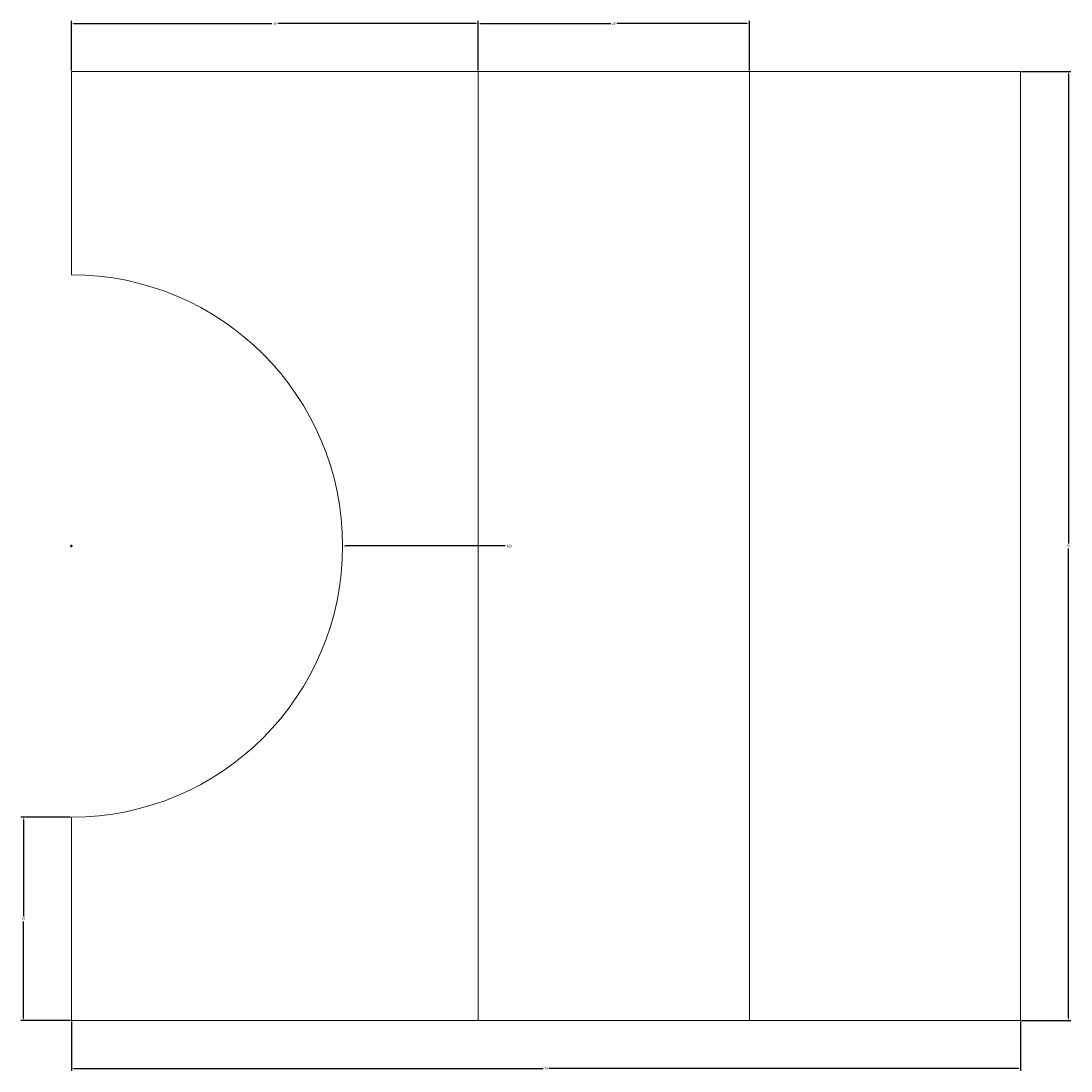
# Model space of a CAD drawing. Units: millimetres. Extents: x 3123.5 to 3200.9, y 1016.4 to 1093.8.
import ezdxf

# ---------------------------------------------------------------- set-up
doc = ezdxf.new("R2010")
doc.units = ezdxf.units.MM
doc.layers.add('M-CONS', color=8, linetype='Continuous', lineweight=13)
doc.layers.add('M-DIMS', color=2, linetype='Continuous', lineweight=18)
doc.styles.get("Standard").update_dxf_attribs({"font": 'arial.ttf'})
doc.dimstyles.get("Standard").update_dxf_attribs({"dimtxt": 0.18, "dimasz": 0.18, "dimexe": 0.18, "dimexo": 0.0625, "dimgap": 0.09, "dimtad": 0, "dimtih": 1, "dimtoh": 1, "dimdec": 4, "dimzin": 0, "dimdsep": 46, "dimtxsty": 'Standard', "dimcen": 0.09, "dimadec": 0, "dimazin": 0, "dimtfac": 1, "dimtdec": 4, "dimtofl": 0, "dimtmove": 0, "dimatfit": 3, "dimfxl": 1, "dimtolj": 1, "dimtzin": 0, "dimarcsym": 0})

# ---------------------------------------------------------------- blocks, each defined once
blk = doc.blocks.new('*D3')
at = {"layer": 'Defpoints', "color": 0, "transparency": 16777216}
for p in [(3127.17, 1020.093), (3197.17, 1020.093), (3197.17, 1016.553)]:
    blk.add_point(p, dxfattribs=at)
at = {"layer": 'M-DIMS', "color": 0, "lineweight": -2, "transparency": 16777216}
for p, q in [((3127.17, 1020.03), (3127.17, 1016.373)), ((3197.17, 1020.03), (3197.17, 1016.373)), ((3127.35, 1016.553), (3161.952, 1016.553)), ((3196.99, 1016.553), (3162.388, 1016.553))]:
    blk.add_line(p, q, dxfattribs=at)
at = {"layer": 'M-DIMS', "color": 0, "transparency": 16777216}
for points in [[(3127.35, 1016.583), (3127.35, 1016.523), (3127.17, 1016.553)], [(3196.99, 1016.583), (3196.99, 1016.523), (3197.17, 1016.553)]]:
    blk.add_solid(points, dxfattribs=at)
at = {"layer": 'M-DIMS', "color": 0, "transparency": 16777216, "insert": (3162.17, 1016.553), "char_height": 0.18, "attachment_point": 5}
blk.add_mtext('\\A1;70', dxfattribs=at)
blk = doc.blocks.new('*D4')
at = {"layer": 'Defpoints', "color": 0, "transparency": 16777216}
for p in [(3197.17, 1090.093), (3200.71, 1090.093), (3197.17, 1020.093)]:
    blk.add_point(p, dxfattribs=at)
at = {"layer": 'M-DIMS', "color": 0, "lineweight": -2, "transparency": 16777216}
for p, q in [((3197.233, 1090.093), (3200.89, 1090.093)), ((3200.71, 1089.913), (3200.71, 1055.275)), ((3200.71, 1020.273), (3200.71, 1054.911)), ((3197.233, 1020.093), (3200.89, 1020.093))]:
    blk.add_line(p, q, dxfattribs=at)
at = {"layer": 'M-DIMS', "color": 0, "transparency": 16777216}
for points in [[(3200.68, 1089.913), (3200.74, 1089.913), (3200.71, 1090.093)], [(3200.68, 1020.273), (3200.74, 1020.273), (3200.71, 1020.093)]]:
    blk.add_solid(points, dxfattribs=at)
at = {"layer": 'M-DIMS', "color": 0, "transparency": 16777216, "insert": (3200.71, 1055.093), "char_height": 0.18, "attachment_point": 5}
blk.add_mtext('\\A1;70', dxfattribs=at)
blk = doc.blocks.new('*D5')
at = {"layer": 'Defpoints', "color": 0, "transparency": 16777216}
for p in [(3157.17, 1093.633), (3127.17, 1090.093), (3157.17, 1090.093)]:
    blk.add_point(p, dxfattribs=at)
at = {"layer": 'M-DIMS', "color": 0, "lineweight": -2, "transparency": 16777216}
for p, q in [((3127.17, 1090.155), (3127.17, 1093.813)), ((3127.35, 1093.633), (3141.952, 1093.633)), ((3156.99, 1093.633), (3142.389, 1093.633)), ((3157.17, 1090.155), (3157.17, 1093.813))]:
    blk.add_line(p, q, dxfattribs=at)
at = {"layer": 'M-DIMS', "color": 0, "transparency": 16777216}
for points in [[(3127.35, 1093.663), (3127.35, 1093.603), (3127.17, 1093.633)], [(3156.99, 1093.663), (3156.99, 1093.603), (3157.17, 1093.633)]]:
    blk.add_solid(points, dxfattribs=at)
at = {"layer": 'M-DIMS', "color": 0, "transparency": 16777216, "insert": (3142.17, 1093.633), "char_height": 0.18, "attachment_point": 5}
blk.add_mtext('\\A1;30', dxfattribs=at)
blk = doc.blocks.new('*D6')
at = {"layer": 'Defpoints', "color": 0, "transparency": 16777216}
for p in [(3177.17, 1093.633), (3157.17, 1090.093), (3177.17, 1090.093)]:
    blk.add_point(p, dxfattribs=at)
at = {"layer": 'M-DIMS', "color": 0, "lineweight": -2, "transparency": 16777216}
for p, q in [((3157.17, 1090.155), (3157.17, 1093.813)), ((3157.35, 1093.633), (3166.95, 1093.633)), ((3176.99, 1093.633), (3167.39, 1093.633)), ((3177.17, 1090.155), (3177.17, 1093.813))]:
    blk.add_line(p, q, dxfattribs=at)
at = {"layer": 'M-DIMS', "color": 0, "transparency": 16777216}
for points in [[(3157.35, 1093.663), (3157.35, 1093.603), (3157.17, 1093.633)], [(3176.99, 1093.663), (3176.99, 1093.603), (3177.17, 1093.633)]]:
    blk.add_solid(points, dxfattribs=at)
at = {"layer": 'M-DIMS', "color": 0, "transparency": 16777216, "insert": (3167.17, 1093.633), "char_height": 0.18, "attachment_point": 5}
blk.add_mtext('\\A1;20', dxfattribs=at)
blk = doc.blocks.new('*D7')
at = {"layer": 'Defpoints', "color": 0, "transparency": 16777216}
for p in [(3123.63, 1035.093), (3127.17, 1035.093), (3127.17, 1020.093)]:
    blk.add_point(p, dxfattribs=at)
at = {"layer": 'M-DIMS', "color": 0, "lineweight": -2, "transparency": 16777216}
for p, q in [((3127.108, 1035.093), (3123.45, 1035.093)), ((3123.63, 1034.913), (3123.63, 1027.775)), ((3123.63, 1020.273), (3123.63, 1027.411)), ((3127.108, 1020.093), (3123.45, 1020.093))]:
    blk.add_line(p, q, dxfattribs=at)
at = {"layer": 'M-DIMS', "color": 0, "transparency": 16777216}
for points in [[(3123.6, 1034.913), (3123.66, 1034.913), (3123.63, 1035.093)], [(3123.6, 1020.273), (3123.66, 1020.273), (3123.63, 1020.093)]]:
    blk.add_solid(points, dxfattribs=at)
at = {"layer": 'M-DIMS', "color": 0, "transparency": 16777216, "insert": (3123.63, 1027.593), "char_height": 0.18, "attachment_point": 5}
blk.add_mtext('\\A1;15', dxfattribs=at)
blk = doc.blocks.new('*D8')
at = {"layer": 'Defpoints', "color": 0, "transparency": 16777216}
for p in [(3127.17, 1055.093), (3147.17, 1055.093)]:
    blk.add_point(p, dxfattribs=at)
at = {"layer": 'M-DIMS', "color": 0, "lineweight": -2, "transparency": 16777216}
for p, q in [((3127.08, 1055.093), (3127.26, 1055.093)), ((3127.17, 1055.003), (3127.17, 1055.183)), ((3159.17, 1055.093), (3147.35, 1055.093))]:
    blk.add_line(p, q, dxfattribs=at)
at = {"layer": 'M-DIMS', "color": 0, "transparency": 16777216}
blk.add_solid([(3147.35, 1055.123), (3147.35, 1055.063), (3147.17, 1055.093)], dxfattribs=at)
at = {"layer": 'M-DIMS', "color": 0, "transparency": 16777216, "insert": (3159.475, 1055.093), "char_height": 0.18, "attachment_point": 5}
blk.add_mtext('\\A1;R20', dxfattribs=at)

msp = doc.modelspace()

# ---------------------------------------------------------------- linework, layer by layer
at = {"layer": 'M-CONS'}
for p, q in [((3197.17, 1090.093, 80), (3177.17, 1090.093, 80)), ((3177.17, 1090.093, 80), (3177.17, 1020.093, 80))]:
    msp.add_line(p, q, dxfattribs=at)
msp.add_lwpolyline([(3197.17, 1020.093), (3127.17, 1020.093), (3127.17, 1035.093, 1), (3127.17, 1075.093), (3127.17, 1090.093), (3197.17, 1090.093), (3197.17, 1020.093), (3157.17, 1020.093), (3157.17, 1090.093)], format="xyb", dxfattribs=at)
at = {"layer": 'M-CONS', "elevation": 60}
msp.add_lwpolyline([(3157.17, 1090.093), (3197.17, 1090.093), (3197.17, 1020.093), (3157.17, 1020.093)], close=True, dxfattribs=at)
at = {"layer": 'M-CONS', "extrusion": (1, 0, 0)}
msp.add_circle((1055.093, 120, 3177.17), 17.5, dxfattribs=at)

# ---------------------------------------------------------------- dimensions: what is measured, and where the dimension line sits
at = {"layer": 'M-DIMS'}
for base, p1, p2, picture, middle in [((3157.17, 1093.633), (3127.17, 1090.093), (3157.17, 1090.093), '*D5', (3142.17, 1093.633)), ((3177.17, 1093.633), (3157.17, 1090.093), (3177.17, 1090.093), '*D6', (3167.17, 1093.633)), ((3197.17, 1016.553), (3127.17, 1020.093), (3197.17, 1020.093), '*D3', (3162.17, 1016.553))]:
    dim = msp.add_linear_dim(base=base, p1=p1, p2=p2, dimstyle='Standard', override={"dimdec": 0, "dimlfac": 1, "dimrnd": 0, "dimzin": 0, "dimdsep": 46, "dimlunit": 2}, dxfattribs=at)
    dim.commit()
    dim.dimension.update_dxf_attribs({"geometry": picture, "text_midpoint": middle})
for base, p1, p2, picture, middle in [((3200.71, 1090.093), (3197.17, 1020.093), (3197.17, 1090.093), '*D4', (3200.71, 1055.093)), ((3123.63, 1035.093), (3127.17, 1020.093), (3127.17, 1035.093), '*D7', (3123.63, 1027.593))]:
    dim = msp.add_linear_dim(base=base, p1=p1, p2=p2, angle=90, dimstyle='Standard', override={"dimdec": 0, "dimlfac": 1, "dimrnd": 0, "dimzin": 0, "dimdsep": 46, "dimlunit": 2}, dxfattribs=at)
    dim.commit()
    dim.dimension.update_dxf_attribs({"geometry": picture, "text_midpoint": middle})
dim = msp.add_radius_dim(center=(3127.17, 1055.093), mpoint=(3147.17, 1055.093), dimstyle='Standard', override={"dimdec": 0, "dimlfac": 1, "dimrnd": 0, "dimzin": 0, "dimdsep": 46, "dimlunit": 2}, dxfattribs=at)
dim.commit()
dim.dimension.update_dxf_attribs({"geometry": '*D8', "text_midpoint": (3159.17, 1055.093), "dimtype": 164})

doc.saveas('drawing.dxf')
